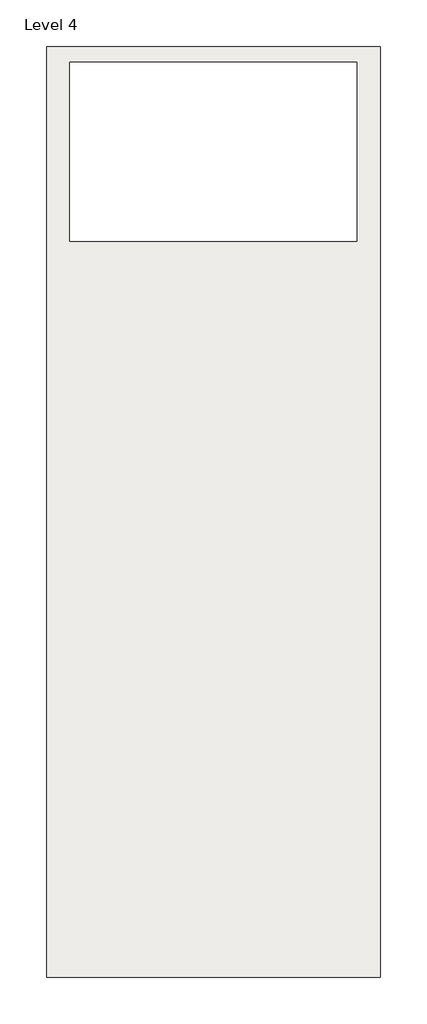
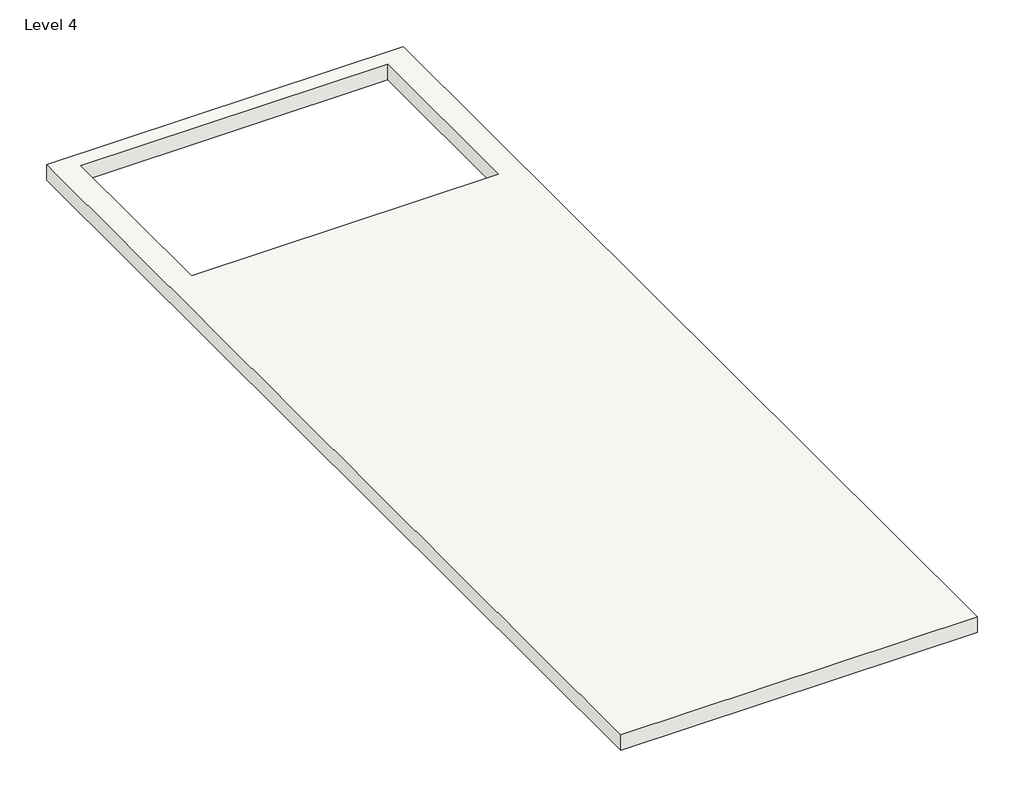
# One storey: 1 slab.
"""IFC4 building model written with IfcOpenShell, lengths in millimetres."""

from ifc_helpers import new_model, si_unit, frame, origin, place, context, project, spatial, polyline, outline, extrude, element, save

model = new_model("IFC4")

# Units and contexts
model_context = context("Model", 3, world=origin())
ifc_project = project(units=[si_unit("LENGTHUNIT", "METRE", prefix="MILLI")], contexts=[model_context])

# Site, building, storey
site = spatial("IfcSite", under=ifc_project)
building = spatial("IfcBuilding", under=site)
storey = spatial("IfcBuildingStorey", under=building, Name="Level 4", Elevation=9601.2)

# Slab
placement = place(None, origin())
element("IfcSlab", 1, ObjectType="6\"", at=placement, inside=storey, context=model_context, shape_type="SweptSolid", body=[
    extrude(outline(polyline([(-3644.6189081, -2293.9597011), (-6921.2189081, -2293.9597011), (-6921.2189081, 6850.0402989), (-3644.6189081, 6850.0402989), (-3644.6189081, -2293.9597011)]), holes=[polyline([(-6692.6189081, 6697.6402989), (-6692.6189081, 4938.1100028), (-3873.2189081, 4938.1100028), (-3873.2189081, 6697.6402989), (-6692.6189081, 6697.6402989)])]), frame((0.0, 0.0, 9448.8), z_axis=(0.0, 0.0, 1.0), x_axis=(1.0, 0.0, 0.0)), (0.0, 0.0, 1.0), 152.4),
])

save(model, "model.ifc")

# Revit data of these elements
# Type "6\""
#   Assembly Code = "B1010"
#   Function = 0
#   Layers, outside or top first: 0' - 6" no material (function 1)
# Element 1 (IfcSlab, "6\"")
#   Height Offset From Level = 0' - 0"
#   Phase Created = New Construction
#   Materials on its faces: "Default Floor"
# Materials
#   "Default Floor": colour RGB 128 128 128, transparency 0
